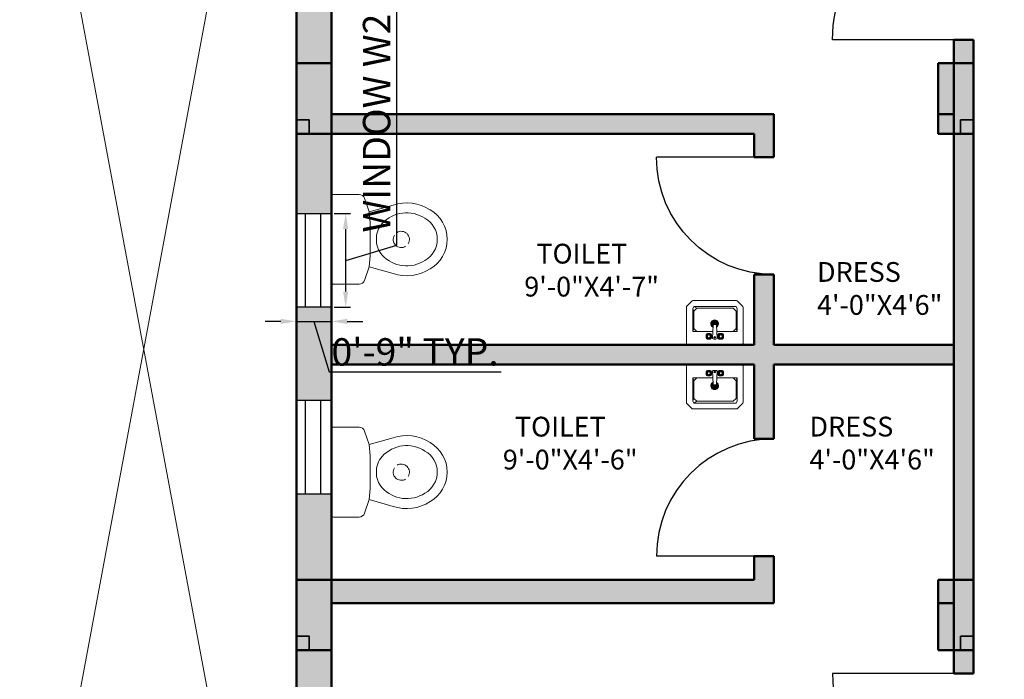
# Model space of a CAD drawing. Units: inches. Extents: x -7 to 1228, y -146 to 1091.
# Tile 26 of 88: x 563 to 815, y 194 to 362. Entities that reach past the tile are written whole.
import ezdxf

# ---------------------------------------------------------------- set-up
doc = ezdxf.new("R2010")
doc.units = ezdxf.units.IN
for name, color, linetype, lineweight in [('A-ANNO-DIMS', 2, 'Continuous', 18), ('A-AREA-IDEN', 7, 'Continuous', 18), ('A-COLS', 6, 'Continuous', 35), ('A-DOOR', 4, 'Continuous', 25), ('A-FLOR-FIXT', 8, 'Continuous', 18), ('A-FLOR-VOID', 7, 'Continuous', 18), ('A-FURN', 8, 'Continuous', 18), ('A-GLAZ', 175, 'Continuous', 25), ('A-WALL', 7, 'Continuous', 50), ('A-WALL-PATT', 251, 'Continuous', 13)]:
    doc.layers.add(name, color=color, linetype=linetype, lineweight=lineweight)
doc.styles.get("Standard").update_dxf_attribs({"font": 'arial.ttf'})
doc.dimstyles.new('ISO-25', dxfattribs={"dimtxt": 7, "dimasz": 4, "dimexe": 1.25, "dimexo": 0.625, "dimtad": 1, "dimdec": 1, "dimlunit": 3, "dimtxsty": 'Standard', "dimcen": 2.5, "dimadec": 0, "dimazin": 0, "dimtfac": 1, "dimtdec": 1, "dimtmove": 1, "dimatfit": 3, "dimfxl": 1, "dimarcsym": 0})

# ---------------------------------------------------------------- blocks, each defined once
blk = doc.blocks.new('A$C7B5C7CD4')
at = {"ltscale": 20}
for p, q in [((0, 0.614), (0, 0.4765)), ((0.243, 0.625), (0.011, 0.625)), ((0.243, 0.625), (0.475, 0.625)), ((0.486, 0.614), (0.486, 0.4765)), ((0.0212, 0.4467), (0.0946, 0.4214)), ((0.4648, 0.4467), (0.3914, 0.4214)), ((0.0946, 0.4214), (0.0576, 0.293)), ((0.0946, 0.4214), (0.1544, 0.4173)), ((0.3316, 0.4173), (0.1544, 0.4173)), ((0.3914, 0.4214), (0.3316, 0.4173)), ((0.3914, 0.4214), (0.4284, 0.293))]:
    blk.add_line(p, q, dxfattribs=at)
for centre, radius, start, end in [((0.011, 0.614), 0.011, 90, 180), ((0.475, 0.614), 0.011, 0, 90), ((0.0315, 0.4765), 0.0315, 180, 251), ((0.4545, 0.4765), 0.0315, 289, 0), ((0.24, 0.2602), 0.123, 88.6158, 131.7414), ((0.246, 0.2602), 0.123, 48.2586, 91.3842), ((0.2796, 0.219), 0.18, 132.4207, 213.289), ((0.2064, 0.219), 0.18, 326.711, 47.5793), ((0.2796, 0.219), 0.234, 161.5846, 212.8753), ((0.2064, 0.219), 0.234, 327.1247, 18.4154), ((0.243, 0.185), 0.131, 209.6292, 270), ((0.243, 0.185), 0.131, 270, 330.3708), ((0.243, 0.185), 0.185, 210.1745, 270), ((0.243, 0.185), 0.185, 270, 329.8255)]:
    blk.add_arc(centre, radius, start, end, dxfattribs=at)
for start, end in [(58.1785, 211.8215), (238.1785, 31.8215)]:
    blk.add_arc((0.2426, 0.2481), 0.0439, start, end)
blk = doc.blocks.new('A$C4CB854FF')
for p, q in [((0, 0.3675), (0, 0.0552)), ((0.4725, 0.38), (0.0125, 0.38)), ((0.485, 0.0552), (0.485, 0.3675)), ((0.05, 0.265), (0.2247, 0.265)), ((0.06, 0.24), (0.05, 0.265)), ((0.05, 0.07), (0.05, 0.265)), ((0.085, 0.265), (0.06, 0.24)), ((0.1677, 0.2932), (0.1677, 0.318)), ((0.1745, 0.2919), (0.1745, 0.3194)), ((0.1773, 0.3221), (0.2048, 0.3221)), ((0.2048, 0.2891), (0.1773, 0.2891)), ((0.1787, 0.329), (0.2034, 0.329)), ((0.2034, 0.2822), (0.1787, 0.2822)), ((0.2075, 0.3194), (0.2075, 0.2919)), ((0.2144, 0.318), (0.2144, 0.2932)), ((0.2279, 0.2104), (0.2213, 0.3235)), ((0.2337, 0.329), (0.2502, 0.329)), ((0.2625, 0.3235), (0.256, 0.2104)), ((0.2591, 0.265), (0.43, 0.265)), ((0.2694, 0.318), (0.2694, 0.2932)), ((0.2763, 0.3194), (0.2763, 0.2919)), ((0.3065, 0.3221), (0.279, 0.3221)), ((0.279, 0.2891), (0.3065, 0.2891)), ((0.3052, 0.329), (0.2804, 0.329)), ((0.2804, 0.2822), (0.3052, 0.2822)), ((0.3093, 0.2919), (0.3093, 0.3194)), ((0.3162, 0.2932), (0.3162, 0.318)), ((0.395, 0.265), (0.42, 0.24)), ((0.42, 0.24), (0.43, 0.265)), ((0.43, 0.07), (0.43, 0.265)), ((0.06, 0.24), (0.06, 0.09)), ((0.2152, 0.1984), (0.2694, 0.1984)), ((0.2297, 0.2066), (0.2165, 0.2066)), ((0.2681, 0.1901), (0.2165, 0.1901)), ((0.2272, 0.2149), (0.2208, 0.2149)), ((0.2638, 0.1819), (0.2208, 0.1819)), ((0.2533, 0.1736), (0.2313, 0.1736)), ((0.2505, 0.2052), (0.2334, 0.2052)), ((0.2681, 0.2066), (0.2541, 0.2066)), ((0.2638, 0.2149), (0.2566, 0.2149)), ((0.42, 0.24), (0.42, 0.09)), ((0.06, 0.09), (0.085, 0.065)), ((0.42, 0.09), (0.395, 0.065)), ((0.42, 0.09), (0.43, 0.07)), ((0.0037, 0.0463), (0.0463, 0.0037)), ((0.05, 0.07), (0.06, 0.05)), ((0.42, 0.05), (0.06, 0.05)), ((0.085, 0.065), (0.395, 0.065)), ((0.395, 0.065), (0.42, 0.05)), ((0.43, 0.07), (0.42, 0.05)), ((0.4387, 0.0037), (0.4813, 0.0463)), ((0.0552, 0), (0.4298, 0))]:
    blk.add_line(p, q)
for centre, radius in [((0.191, 0.3056), 0.0165), ((0.191, 0.3056), 0.0127), ((0.2419, 0.3152), 0.00688), ((0.2419, 0.3152), 0.00344), ((0.2928, 0.3056), 0.0165), ((0.2928, 0.3056), 0.0127)]:
    blk.add_circle(centre, radius)
for centre, radius, start, end in [((0.0125, 0.3675), 0.0125, 90, 180), ((0.4725, 0.3675), 0.0125, 0, 90), ((0.1787, 0.318), 0.011, 90, 180), ((0.1787, 0.2932), 0.011, 180, 270), ((0.1773, 0.3194), 0.00275, 90, 180), ((0.1773, 0.2919), 0.00275, 180, 270), ((0.2034, 0.318), 0.011, 0, 90), ((0.2034, 0.2932), 0.011, 270, 0), ((0.2048, 0.3194), 0.00275, 360, 90), ((0.2048, 0.2919), 0.00275, 270, 0), ((0.2329, 0.314), 0.015, 87.19754, 140.72744), ((0.2509, 0.314), 0.015, 39.27256, 92.80246), ((0.2804, 0.318), 0.011, 90, 180), ((0.2804, 0.2932), 0.011, 180, 270), ((0.279, 0.3194), 0.00275, 90, 180), ((0.279, 0.2919), 0.00275, 180, 270), ((0.3052, 0.318), 0.011, 0, 90), ((0.3052, 0.2932), 0.011, 270, 360), ((0.3065, 0.3194), 0.00275, 360, 90), ((0.3065, 0.2919), 0.00275, 270, 0), ((0.2423, 0.1984), 0.033, 118.68833, 62.86857), ((0.2423, 0.1984), 0.0271, 124.77581, 57.22467), ((0.2334, 0.2107), 0.0055, 183.3274, 270), ((0.2505, 0.2107), 0.0055, 270, 356.6726), ((0.0125, 0.0552), 0.0125, 180, 225), ((0.0552, 0.0125), 0.0125, 225, 270), ((0.4298, 0.0125), 0.0125, 270, 315), ((0.4725, 0.0552), 0.0125, 315, 0)]:
    blk.add_arc(centre, radius, start, end)
blk = doc.blocks.new('WIN-24')
for p, q in [((0, 0), (0, 24)), ((0, 24), (9, 24)), ((2.34, 0), (2.34, 24)), ((2.34, 24), (6.14, 24)), ((6.14, 24), (6.14, 0)), ((9, 24), (9, 0)), ((9, 0), (0, 0))]:
    blk.add_line(p, q)
blk = doc.blocks.new('DOOR-750')
blk.add_line((30, 30), (30, 0))
blk.add_arc((30, 30), 30, 180, 270)
blk = doc.blocks.new('DOOR-900')
blk.add_line((36, 0), (36, 36))
blk.add_arc((36, 0), 36, 90, 180)
blk = doc.blocks.new('*D50')
at = {"layer": 'A-ANNO-DIMS', "color": 0, "lineweight": -2, "transparency": 16777216}
for p, q in [((659.65, 304.55), (659.65, 411.76)), ((643.62, 312.63), (647.85, 312.63)), ((646.6, 292.63), (646.6, 308.63)), ((646.6, 300.63), (659.65, 304.55)), ((643.62, 288.63), (647.85, 288.63))]:
    blk.add_line(p, q, dxfattribs=at)
at = {"layer": 'A-ANNO-DIMS', "color": 0, "transparency": 16777216}
for points in [[(645.93, 308.63), (647.27, 308.63), (646.6, 312.63)], [(645.93, 292.63), (647.27, 292.63), (646.6, 288.63)]]:
    blk.add_solid(points, dxfattribs=at)
at = {"layer": 'Defpoints', "color": 0, "transparency": 16777216}
for p in [(643, 312.63), (646.6, 312.63), (643, 288.63)]:
    blk.add_point(p, dxfattribs=at)
at = {"layer": 'A-ANNO-DIMS', "color": 0, "transparency": 16777216, "insert": (655.41, 358.15), "char_height": 7, "attachment_point": 5, "rotation": 90}
blk.add_mtext('WINDOW W2 2\'-0" TYP.', dxfattribs=at)
blk = doc.blocks.new('*D51')
at = {"layer": 'A-ANNO-DIMS', "color": 0, "lineweight": -2, "transparency": 16777216}
for p, q in [((634, 288), (634, 283.78)), ((643, 288), (643, 283.78)), ((630, 285.03), (626, 285.03)), ((634, 285.03), (643, 285.03)), ((634, 285.03), (643, 285.03)), ((638.5, 285.03), (642.37, 272.12)), ((647, 285.03), (651, 285.03)), ((642.37, 272.12), (686.29, 272.12))]:
    blk.add_line(p, q, dxfattribs=at)
at = {"layer": 'A-ANNO-DIMS', "color": 0, "transparency": 16777216}
for points in [[(630, 285.7), (630, 284.36), (634, 285.03)], [(647, 285.7), (647, 284.36), (643, 285.03)]]:
    blk.add_solid(points, dxfattribs=at)
at = {"layer": 'Defpoints', "color": 0, "transparency": 16777216}
for p in [(634, 288.63), (643, 288.63), (643, 285.03)]:
    blk.add_point(p, dxfattribs=at)
at = {"layer": 'A-ANNO-DIMS', "color": 0, "transparency": 16777216, "insert": (664.33, 276.32), "char_height": 7, "attachment_point": 5}
blk.add_mtext('0\'-9" TYP.', dxfattribs=at)

msp = doc.modelspace()

# ---------------------------------------------------------------- hatches: boundary and pattern name
at = {"layer": 'A-COLS'}
h = msp.add_hatch(color=256, dxfattribs=at)
h.dxf.hatch_style = 1
h.paths.add_polyline_path([(634, 336.55), (637.29, 336.55), (637.29, 333), (643, 333), (643, 351), (634, 351)])
h = msp.add_hatch(color=256, dxfattribs=at)
h.dxf.hatch_style = 1
h.paths.add_polyline_path([(807, 351), (798, 351), (798, 333), (803.71, 333), (803.71, 336.55), (807, 336.55)])
h = msp.add_hatch(color=256, dxfattribs=at)
h.dxf.hatch_style = 1
h.paths.add_polyline_path([(634, 336.55), (634, 333), (637.29, 333), (637.29, 336.55)])
h = msp.add_hatch(color=256, dxfattribs=at)
h.dxf.hatch_style = 1
h.paths.add_polyline_path([(803.71, 336.55), (803.71, 333), (807, 333), (807, 336.55)])
h = msp.add_hatch(color=256, dxfattribs=at)
h.dxf.hatch_style = 1
h.paths.add_polyline_path([(634, 204.55), (637.29, 204.55), (637.29, 201), (643, 201), (643, 219), (634, 219)])
h = msp.add_hatch(color=256, dxfattribs=at)
h.dxf.hatch_style = 1
h.paths.add_polyline_path([(807, 219), (798, 219), (798, 201), (803.71, 201), (803.71, 204.55), (807, 204.55)])
h = msp.add_hatch(color=256, dxfattribs=at)
h.dxf.hatch_style = 1
h.paths.add_polyline_path([(634, 204.55), (634, 201), (637.29, 201), (637.29, 204.55)])
h = msp.add_hatch(color=256, dxfattribs=at)
h.dxf.hatch_style = 1
h.paths.add_polyline_path([(803.71, 204.55), (803.71, 201), (807, 201), (807, 204.55)])
at = {"layer": 'A-WALL-PATT'}
h = msp.add_hatch(color=256, dxfattribs=at)
h.dxf.hatch_style = 1
h.paths.add_polyline_path([(69, 568), (60, 568), (60, 493), (63.29, 493), (69, 493)])
h.paths.add_polyline_path([(69, 662.41), (60, 662.41), (60, 586), (69, 586)], flags=17)
h.paths.add_polyline_path([(69, 723), (184, 723), (184, 734), (179, 734), (179, 728), (69, 728), (69, 741.62), (60, 741.62), (60, 698.41), (69, 698.41)], flags=17)
h.paths.add_polyline_path([(69, 782), (231, 782), (231, 728), (231, 723), (231, 586), (236, 586), (236, 787), (69, 787), (69, 800.13), (60, 800.13), (60, 765.62), (69, 765.62)])
h.paths.add_polyline_path([(184, 842), (189, 842), (189, 848), (173, 848), (173, 842), (179, 842), (179, 787), (184, 787)])
h.paths.add_polyline_path([(118.22, 69), (69, 69), (69, 60), (118.22, 60)])
h.paths.add_polyline_path([(227, 69), (154.22, 69), (154.22, 60), (227, 60)])
h.paths.add_polyline_path([(236, 60), (232.71, 60), (227, 60), (227, 36), (236, 36)])
h.paths.add_polyline_path([(389, 60), (380, 60), (380, 36), (389, 36)])
h.paths.add_polyline_path([(384, 181), (380, 181), (380, 115), (380, 78), (384, 78)])
h.paths.add_polyline_path([(380, 115), (334.55, 115), (334.55, 109), (380, 109)])
h.paths.add_polyline_path([(274.55, 115), (236, 115), (236, 201), (232.71, 201), (231, 201), (231, 78), (236, 78), (236, 109), (274.55, 109)])
h.paths.add_polyline_path([(69, 123), (60, 123), (60, 78), (69, 78)])
h.paths.add_polyline_path([(69, 201), (60, 201), (60, 159), (69, 159)])
h.paths.add_polyline_path([(143, 219), (69, 219), (69, 213), (143, 213)], flags=17)
h.paths.add_polyline_path([(189, 219), (184, 219), (184, 274), (231, 274), (231, 219), (236, 219), (236, 279), (184, 279), (184, 297), (179, 297), (179, 279), (69, 279), (69, 290.91), (60, 290.91), (60, 262.18), (69, 262.18), (69, 274), (179, 274), (179, 219), (173, 219), (173, 213), (189, 213)])
h.paths.add_polyline_path([(69, 238.18), (60, 238.18), (60, 219), (69, 219)], flags=17)
h.paths.add_polyline_path([(69, 333), (60, 333), (60, 314.91), (69, 314.91), (69, 316.96)])
h.paths.add_polyline_path([(190, 338), (184, 338), (69, 338), (69, 333), (179, 333), (179, 327), (184, 327), (184, 333.02), (190, 333.05)])
h.paths.add_polyline_path([(69, 386.81), (60, 386.81), (60, 351), (69, 351)])
h.paths.add_polyline_path([(69, 475), (60, 475), (60, 422.81), (69, 422.81)])
h.paths.add_polyline_path([(236, 475), (231, 475), (231, 351.24), (236, 351.24)])
h.paths.add_polyline_path([(384, 475), (380, 475), (380, 362), (384, 362)])
h.paths.add_polyline_path([(547, 307), (439, 307), (439, 356), (445, 356), (445, 362), (433, 362), (433, 307), (380, 307), (380, 244), (380, 241), (384, 241), (384, 301), (433, 301), (433, 277), (439, 277), (439, 301), (547, 301)])
h.paths.add_polyline_path([(547, 241), (439, 241), (439, 247), (433, 247), (433, 235), (547, 235)])
h.paths.add_polyline_path([(450, 69), (440.29, 69), (424.89, 69), (389, 69), (389, 60), (450, 60)])
h.paths.add_polyline_path([(547, 69), (486, 69), (486, 60), (547, 60)])
h.paths.add_polyline_path([(556, 148.27), (547, 148.27), (547, 78), (556, 78)])
h.paths.add_polyline_path([(556, 223), (547, 223), (547, 195), (547, 184.27), (556, 184.27)])
h.paths.add_polyline_path([(556, 311.19), (547, 311.19), (547, 273.08), (556, 273.08)])
h.paths.add_polyline_path([(556, 344), (552.71, 344), (547, 344), (547, 335.19), (556, 335.19)])
h.paths.add_polyline_path([(556, 249.08), (547, 249.08), (547, 241), (556, 241)])
h.paths.add_polyline_path([(547, 362), (475, 362), (475, 356), (547, 356)], flags=0)
h.paths.add_polyline_path([(556, 399.62), (547, 399.62), (547, 362), (556, 362)])
h.paths.add_polyline_path([(556, 475), (547, 475), (547, 435.62), (556, 435.62)])
h.paths.add_polyline_path([(547, 493), (389, 493), (389, 487), (547, 487)])
h.paths.add_polyline_path([(380, 493), (278, 493), (278, 487), (380, 487)])
h.paths.add_polyline_path([(227, 493), (69, 493), (69, 487), (227, 487)])
h.paths.add_polyline_path([(643, 122.44), (634, 122.44), (634, 78), (643, 78)])
h.paths.add_polyline_path([(702.5, 69), (692.79, 69), (677.39, 69), (643, 69), (643, 60), (702.5, 60)])
h.paths.add_polyline_path([(798, 69), (738.5, 69), (738.5, 60), (798, 60)])
h.paths.add_polyline_path([(807, 60), (803.71, 60), (798, 60), (798, 36), (807, 36)])
h.paths.add_polyline_path([(807, 109), (846.75, 109), (846.75, 115), (807, 115), (807, 159), (802, 159), (802, 78), (807, 78)])
h.paths.add_polyline_path([(807, 201), (802, 201), (802, 195), (807, 195)])
h.paths.add_polyline_path([(643, 201), (634, 201), (634, 158.44), (643, 158.44)])
h.paths.add_polyline_path([(756, 225), (751, 225), (751, 219), (643, 219), (643, 213), (756, 213)])
h.paths.add_polyline_path([(643, 240.85), (634, 240.85), (634, 219), (643, 219)])
h.paths.add_polyline_path([(643, 274), (643, 288.63), (634, 288.63), (634, 264.85), (643, 264.85)])
h.paths.add_polyline_path([(802, 279), (756, 279), (756, 297), (751, 297), (751, 279), (643, 279), (643, 274), (751, 274), (751, 255), (756, 255), (756, 274), (802, 274)])
h.paths.add_polyline_path([(807, 333), (803.71, 333), (802, 333), (802, 279), (802, 274), (802, 219), (807, 219)])
h.paths.add_polyline_path([(956, 182), (951, 182), (951, 115), (906.75, 115), (906.75, 109), (951, 109), (951, 78), (956, 78)])
h.paths.add_polyline_path([(960, 60), (951, 60), (951, 36), (960, 36)])
h.paths.add_polyline_path([(1021, 69), (1005.78, 69), (960, 69), (960, 60), (1021, 60)])
h.paths.add_polyline_path([(956, 224), (951, 224), (951, 218), (956, 218)])
h.paths.add_polyline_path([(956, 302), (1004, 302), (1004, 278), (1010, 278), (1010, 302), (1118, 302), (1118, 290.81), (1127, 290.81), (1127, 326.97), (1118, 326.97), (1118, 320.97), (1118, 307), (1010, 307), (1010, 356), (1016, 356), (1016, 362), (1004, 362), (1004, 307), (951, 307), (951, 244), (951, 242), (954.29, 242), (956, 242)])
h.paths.add_polyline_path([(643, 333), (634, 333), (634, 312.63), (643, 312.63), (643, 316.96)])
h.paths.add_polyline_path([(756, 338), (643, 338), (643, 333), (751, 333), (751, 327), (756, 327)])
h.paths.add_polyline_path([(643, 388), (634, 388), (634, 351), (643, 351)])
h.paths.add_polyline_path([(807, 357), (802, 357), (802, 351), (807, 351)])
h.paths.add_polyline_path([(807, 475), (802, 475), (802, 393), (807, 393)])
h.paths.add_polyline_path([(643, 475), (634, 475), (634, 424), (643, 424)])
h.paths.add_polyline_path([(798, 493), (643, 493), (643, 487), (798, 487)])
h.paths.add_polyline_path([(634, 493), (556, 493), (556, 487), (634, 487)])
h.paths.add_polyline_path([(813, 493), (807, 493), (807, 487), (813, 487)])
h.paths.add_polyline_path([(951, 493), (849, 493), (849, 487), (951, 487)])
h.paths.add_polyline_path([(956, 484), (951, 484), (951, 374), (956, 374)])
h.paths.add_polyline_path([(1109, 493), (969, 493), (969, 487), (1109, 487)])
h.paths.add_polyline_path([(1127, 484), (1118, 484), (1118, 450.64), (1127, 450.64)])
h.paths.add_polyline_path([(1127, 414.64), (1118, 414.64), (1118, 365), (1127, 365)])
h.paths.add_polyline_path([(1109, 362), (1046, 362), (1046, 356), (1109, 356)], flags=17)
h.paths.add_polyline_path([(1127, 356), (1123.45, 356), (1118, 356), (1118, 350.97), (1127, 350.97)], flags=0)
h.paths.add_polyline_path([(1127, 266.81), (1118, 266.81), (1118, 262.36), (1118, 242), (1127, 242)], flags=17)
h.paths.add_polyline_path([(1118, 242), (1010, 242), (1010, 248), (1004, 248), (1004, 237), (1118, 237)])
h.paths.add_polyline_path([(1127, 224), (1118, 224), (1118, 170), (1127, 170)])
h.paths.add_polyline_path([(1127, 134), (1118, 134), (1118, 78), (1127, 78)])
h.paths.add_polyline_path([(1118, 69), (1057, 69), (1057, 60), (1118, 60)])
h.paths.add_polyline_path([(227, 571.55), (227, 574), (69, 574), (69, 568), (227, 568)])
h.paths.add_polyline_path([(380, 571.55), (380, 574), (278, 574), (278, 568), (380, 568)])
h.paths.add_polyline_path([(242, 574), (236, 574), (236, 568), (242, 568)])
h.paths.add_polyline_path([(547, 571.55), (547, 574), (389, 574), (389, 568), (547, 568)])
h.paths.add_polyline_path([(384, 733), (380, 733), (380, 586), (384, 586)])
h.paths.add_polyline_path([(556, 646), (634, 646), (634, 655), (547, 655), (547, 586), (556, 586)])
h.paths.add_polyline_path([(634, 574), (556, 574), (556, 568), (634, 568)])
h.paths.add_polyline_path([(643, 655), (634, 655), (634, 586), (643, 586)])
h.paths.add_polyline_path([(798, 574), (643, 574), (643, 568), (798, 568)])
h.paths.add_polyline_path([(643, 663.85), (634, 663.85), (634, 655), (643, 655)])
h.paths.add_polyline_path([(556, 676.97), (547, 676.97), (547, 655), (556, 655)])
h.paths.add_polyline_path([(556, 733), (547, 733), (547, 712.97), (556, 712.97)])
h.paths.add_polyline_path([(643, 710), (634, 710), (634, 699.85), (643, 699.85)])
h.paths.add_polyline_path([(807, 668), (802, 668), (802, 586), (807, 586)])
h.paths.add_polyline_path([(951, 574), (849, 574), (849, 568), (951, 568)])
h.paths.add_polyline_path([(956, 691), (951, 691), (951, 577), (956, 577)])
h.paths.add_polyline_path([(1109, 574), (969, 574), (969, 568), (1109, 568)])
h.paths.add_polyline_path([(1127, 643.4), (1118, 643.4), (1118, 577), (1127, 577)])
h.paths.add_polyline_path([(1127, 568), (1123.45, 568), (1118, 568), (1118, 493), (1127, 493)])
h.paths.add_polyline_path([(1127, 733), (1118, 733), (1118, 679.4), (1127, 679.4)])
h.paths.add_polyline_path([(1127, 777.35), (1118, 777.35), (1118, 770.04), (1118, 751), (1127, 751)], flags=17)
h.paths.add_polyline_path([(1118, 751), (1010, 751), (1010, 757), (1004, 757), (1004, 745), (1118, 745)])
h.paths.add_polyline_path([(956, 811), (1004, 811), (1004, 787), (1010, 787), (1010, 811), (1017.87, 811), (1017.87, 811.63, -0.414214), (1018.25, 812), (1031.98, 812, -0.414214), (1032.35, 811.63), (1032.35, 811), (1118, 811), (1118, 801.35), (1127, 801.35), (1127, 834.69), (1118, 834.69), (1118, 830.24), (1118, 817), (1010, 817), (1010, 866), (1016, 866), (1016, 872), (1004, 872), (1004, 817), (956, 817), (956, 866), (951, 866), (951, 751), (954.29, 751), (956, 751)])
h.paths.add_polyline_path([(1118, 872), (1046, 872), (1046, 866), (1118, 866)], flags=17)
h.paths.add_polyline_path([(1127, 924.71), (1118, 924.71), (1118, 884), (1127, 884)])
h.paths.add_polyline_path([(1127, 866), (1123.71, 866), (1118, 866), (1118, 858.69), (1127, 858.69)], flags=17)
h.paths.add_polyline_path([(956, 983), (951, 983), (951, 952), (807, 952), (807, 983), (802, 983), (802, 902), (807, 902), (807, 946), (951, 946), (951, 884), (956, 884)])
h.paths.add_polyline_path([(807, 842), (802, 842), (802, 787), (756, 787), (756, 806), (751, 806), (751, 787), (643, 787), (643, 782), (751, 782), (751, 764), (756, 764), (756, 782), (802, 782), (802, 728), (807, 728)])
h.paths.add_polyline_path([(756, 848), (643, 848), (643, 842), (751, 842), (751, 836), (756, 836)])
h.paths.add_polyline_path([(756, 734), (751, 734), (751, 728), (643, 728), (643, 723), (756, 723)])
h.paths.add_polyline_path([(643, 749.79), (634, 749.79), (634, 728), (637.29, 728), (643, 728)])
h.paths.add_polyline_path([(643, 805.41), (634, 805.41), (634, 773.79), (643, 773.79)])
h.paths.add_polyline_path([(643, 896.66), (634, 896.66), (634, 860), (637.29, 860), (643, 860)])
h.paths.add_polyline_path([(643, 842), (634, 842), (634, 829.41), (643, 829.41)])
h.paths.add_polyline_path([(643, 983), (634, 983), (634, 932.66), (643, 932.66)])
h.paths.add_polyline_path([(1127, 983), (1118, 983), (1118, 960.71), (1127, 960.71)])
h.paths.add_polyline_path([(1118, 1001), (1077.53, 1001), (1077.53, 992), (1118, 992)])
h.paths.add_polyline_path([(1041.53, 1001), (960, 1001), (960, 992), (1041.53, 992)])
h.paths.add_polyline_path([(960, 1025), (951, 1025), (951, 1001), (954.29, 1001), (960, 1001)])
h.paths.add_polyline_path([(807, 1025), (798, 1025), (798, 1001), (807, 1001)])
h.paths.add_polyline_path([(798, 1001), (738.5, 1001), (738.5, 992), (798, 992)])
h.paths.add_polyline_path([(702.5, 1001), (643, 1001), (643, 992), (702.5, 992)])
h.paths.add_polyline_path([(547, 1001), (499.11, 1001), (499.11, 992), (547, 992)])
h.paths.add_polyline_path([(463.11, 1001), (389, 1001), (389, 992), (463.11, 992)])
h.paths.add_polyline_path([(389, 1025), (380, 1025), (380, 1022), (380, 1001), (383.29, 1001), (389, 1001)])
h.paths.add_polyline_path([(236, 1025), (227, 1025), (227, 1001), (236, 1001)])
h.paths.add_polyline_path([(236, 983), (231, 983), (231, 860), (236, 860)])
h.paths.add_polyline_path([(274.55, 952), (236, 952), (236, 946), (274.55, 946)])
h.paths.add_polyline_path([(380, 952), (334.55, 952), (334.55, 946), (380, 946)])
h.paths.add_polyline_path([(384, 983), (380, 983), (380, 884), (383.29, 884), (384, 884)])
h.paths.add_polyline_path([(227, 1001), (155.01, 1001), (155.01, 992), (162.87, 992), (227, 992)])
h.paths.add_polyline_path([(119.01, 1001), (69, 1001), (69, 992), (119.01, 992)])
h.paths.add_polyline_path([(69, 983), (60, 983), (60, 922.99), (69, 922.99)])
h.paths.add_polyline_path([(69, 886.99), (60, 886.99), (60, 860), (63.29, 860), (69, 860)])
h.paths.add_polyline_path([(143, 848), (69, 848), (69, 842), (143, 842)])

# ---------------------------------------------------------------- linework, layer by layer
at = {"layer": 'A-COLS'}
for points in [[(634, 333), (637.29, 333), (637.29, 336.55), (634, 336.55)], [(807, 333), (803.71, 333), (803.71, 336.55), (807, 336.55)], [(634, 201), (637.29, 201), (637.29, 204.55), (634, 204.55)], [(807, 201), (803.71, 201), (803.71, 204.55), (807, 204.55)]]:
    msp.add_lwpolyline(points, close=True, dxfattribs=at)
at = {"layer": 'A-FLOR-VOID'}
for p, q in [((634, 487), (556, 69)), ((556, 487), (634, 69))]:
    msp.add_line(p, q, dxfattribs=at)
at = {"layer": 'A-WALL'}
for p, q in [((634, 493), (634, 60)), ((643, 338), (643, 493)), ((643, 493), (643, 60)), ((634, 60), (634, 406)), ((802, 338), (802, 357)), ((807, 357), (802, 357)), ((802, 357), (802, 195)), ((807, 195), (807, 357)), ((807, 357), (807, 195)), ((643, 351), (634, 351)), ((634, 351), (634, 333)), ((643, 333), (643, 351)), ((643, 351), (643, 345)), ((798, 333), (798, 351)), ((798, 351), (807, 351)), ((807, 351), (807, 333)), ((756, 338), (643, 338)), ((756, 327), (756, 338)), ((802, 338), (798, 338)), ((634, 333), (643, 333)), ((751, 333), (643, 333)), ((643, 279), (643, 333)), ((751, 327), (751, 333)), ((802, 333), (798, 333)), ((807, 333), (798, 333)), ((802, 279), (802, 333)), ((756, 327), (751, 327)), ((751, 279), (751, 297)), ((756, 297), (751, 297)), ((756, 279), (756, 297)), ((751, 279), (643, 279)), ((802, 279), (756, 279)), ((751, 274), (643, 274)), ((643, 219), (643, 274)), ((751, 255), (751, 274)), ((802, 274), (756, 274)), ((756, 255), (756, 274)), ((802, 219), (802, 274)), ((756, 255), (751, 255)), ((751, 219), (751, 225)), ((756, 225), (751, 225)), ((756, 213), (756, 225)), ((643, 219), (634, 219)), ((634, 219), (634, 201)), ((751, 219), (643, 219)), ((643, 201), (643, 219)), ((643, 219), (643, 213)), ((802, 219), (798, 219)), ((798, 201), (798, 219)), ((798, 219), (807, 219)), ((807, 219), (807, 201)), ((756, 213), (643, 213)), ((643, 60), (643, 213)), ((802, 213), (798, 213)), ((802, 195), (802, 213)), ((634, 201), (643, 201)), ((807, 201), (798, 201)), ((807, 201), (802, 201)), ((807, 195), (802, 195))]:
    msp.add_line(p, q, dxfattribs=at)

# ---------------------------------------------------------------- block references
at = {"layer": 'A-DOOR', "extrusion": (0, 0, -1), "zscale": -1}
for name, p, rotation in [('DOOR-900', (-807, 393), 269.9999999999997), ('DOOR-750', (-726, 297), 90.00000000000006)]:
    msp.add_blockref(name, p, dxfattribs=dict(at, rotation=rotation))
at = {"layer": 'A-DOOR'}
for name, p, rotation in [('DOOR-750', (726, 255), 270), ('DOOR-900', (807, 159), 89.99999999999969)]:
    msp.add_blockref(name, p, dxfattribs=dict(at, rotation=rotation))
at = {"layer": 'A-FLOR-FIXT', "xscale": 47.26153857112405, "yscale": 47.26153857112405, "zscale": 47.26153857112405, "rotation": 90}
for p in [(672.54, 294.52), (672.54, 235.02)]:
    msp.add_blockref('A$C7B5C7CD4', p, dxfattribs=at)
at = {"layer": 'A-FURN', "xscale": 29.84864686937646, "yscale": 29.84864686937646, "zscale": 29.84864686937646, "rotation": 180}
msp.add_blockref('A$C4CB854FF', (748.13, 290.34), dxfattribs=at)
at = {"layer": 'A-FURN', "xscale": -29.84864686937646, "yscale": 29.84864686937646, "zscale": 29.84864686937646}
msp.add_blockref('A$C4CB854FF', (748.13, 262.66), dxfattribs=at)
at = {"layer": 'A-GLAZ'}
for p in [(634, 288.63), (634, 240.85)]:
    msp.add_blockref('WIN-24', p, dxfattribs=at)

# ---------------------------------------------------------------- texts
at = {"layer": 'A-AREA-IDEN', "attachment_point": 1}
for s, insert, char_height in [('  TOILET\\P9\'-0"X4\'-7"', (692.23, 304.87), 5.0568), ('DRESS\\P4\'-0"X4\'6"', (767.03, 300.19), 5.057), ('  TOILET\\P9\'-0"X4\'-6"', (686.75, 260.65), 5.0568), ('DRESS\\P4\'-0"X4\'6"', (765.1, 260.66), 5.057)]:
    msp.add_mtext_dynamic_manual_height_columns(s, width=137.2821, gutter_width=25.28, heights=[0], dxfattribs=dict(at, insert=insert, char_height=char_height))

# ---------------------------------------------------------------- dimensions: what is measured, and where the dimension line sits
at = {"layer": 'A-ANNO-DIMS'}
dim = msp.add_linear_dim(base=(646.6, 312.63), p1=(643, 288.63), p2=(643, 312.63), angle=90, text='WINDOW W2 <> TYP.', dimstyle='ISO-25', override={"dimdec": 1, "dimlfac": 1, "dimrnd": 0, "dimzin": 1, "dimdsep": 46, "dimlunit": 4, "dimfrac": 2}, dxfattribs=at)
dim.commit()
dim.dimension.update_dxf_attribs({"geometry": '*D50', "text_midpoint": (655.41, 305.17)})
dim = msp.add_linear_dim(base=(643, 285.03), p1=(634, 288.63), p2=(643, 288.63), text='<> TYP.', dimstyle='ISO-25', override={"dimdec": 1, "dimlfac": 1, "dimrnd": 0, "dimzin": 1, "dimdsep": 46, "dimlunit": 4, "dimfrac": 2}, dxfattribs=at)
dim.commit()
dim.dimension.update_dxf_attribs({"geometry": '*D51', "text_midpoint": (643, 276.32)})

doc.saveas('drawing.dxf')
